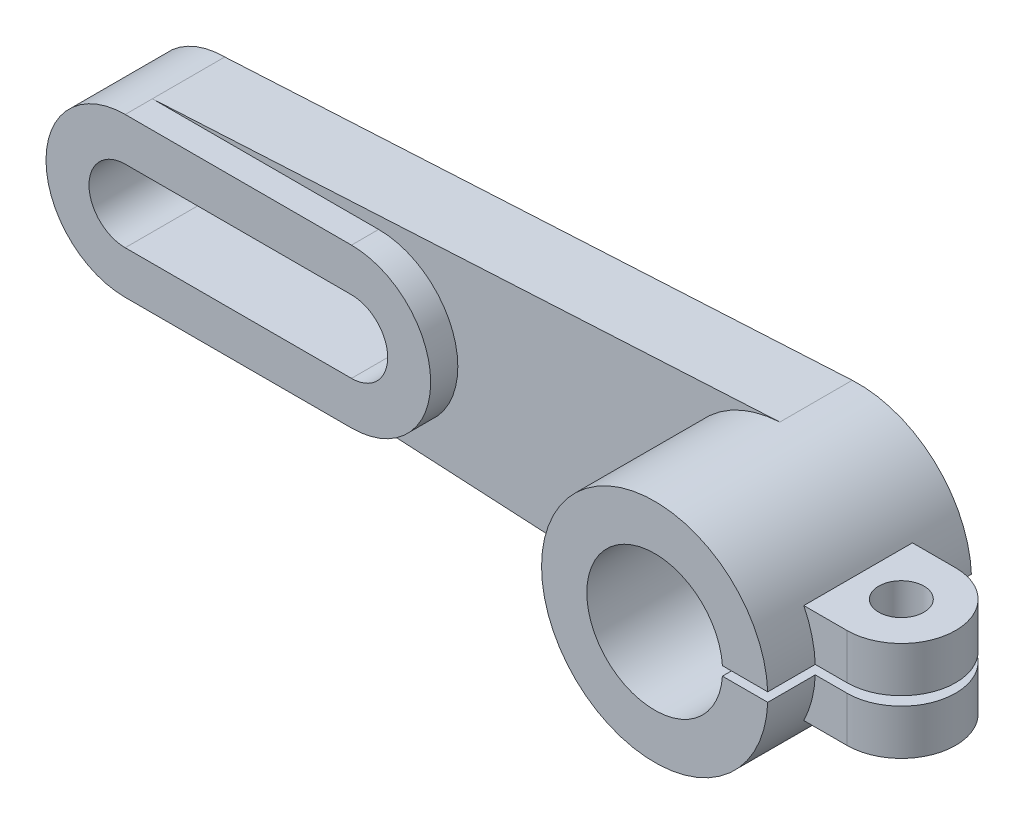
ISO-10303-21;
HEADER;
FILE_DESCRIPTION(('STEP AP214'),'2;1');
FILE_NAME('part.step','',(''),(''),'','','');
FILE_SCHEMA(('AUTOMOTIVE_DESIGN { 1 0 10303 214 1 1 1 1 }'));
ENDSEC;
DATA;
#1=APPLICATION_CONTEXT('core data for automotive mechanical design processes');
#2=APPLICATION_PROTOCOL_DEFINITION('international standard','automotive_design',2000,#1);
#3=PRODUCT_CONTEXT('',#1,'mechanical');
#4=PRODUCT('Part','Part','',(#3));
#5=PRODUCT_RELATED_PRODUCT_CATEGORY('part','',(#4));
#6=PRODUCT_DEFINITION_FORMATION('','',#4);
#7=PRODUCT_DEFINITION_CONTEXT('part definition',#1,'design');
#8=PRODUCT_DEFINITION('design','',#6,#7);
#9=PRODUCT_DEFINITION_SHAPE('','',#8);
#10=(LENGTH_UNIT() NAMED_UNIT(*) SI_UNIT(.MILLI.,.METRE.));
#11=(NAMED_UNIT(*) PLANE_ANGLE_UNIT() SI_UNIT($,.RADIAN.));
#12=(NAMED_UNIT(*) SI_UNIT($,.STERADIAN.) SOLID_ANGLE_UNIT());
#13=UNCERTAINTY_MEASURE_WITH_UNIT(LENGTH_MEASURE(1.E-05),#10,'distance_accuracy_value','');
#14=(GEOMETRIC_REPRESENTATION_CONTEXT(3) GLOBAL_UNCERTAINTY_ASSIGNED_CONTEXT((#13)) GLOBAL_UNIT_ASSIGNED_CONTEXT((#10,
#11,#12)) REPRESENTATION_CONTEXT('',''));
#15=CARTESIAN_POINT('',(0.,0.,0.));
#16=DIRECTION('',(0.,0.,1.));
#17=DIRECTION('',(1.,0.,0.));
#18=AXIS2_PLACEMENT_3D('',#15,#16,#17);
#19=CARTESIAN_POINT('',(32.,11.,22.5));
#20=DIRECTION('',(0.,-1.,0.));
#21=DIRECTION('',(0.,0.,-1.));
#22=AXIS2_PLACEMENT_3D('',#19,#20,#21);
#23=CYLINDRICAL_SURFACE('',#22,12.);
#24=DIRECTION('',(0.,-1.,0.));
#25=VECTOR('',#24,1.);
#26=CARTESIAN_POINT('',(32.,11.,10.5));
#27=LINE('',#26,#25);
#28=CARTESIAN_POINT('',(32.,-1.,10.5));
#29=VERTEX_POINT('',#28);
#30=CARTESIAN_POINT('',(32.,-11.,10.5));
#31=VERTEX_POINT('',#30);
#32=EDGE_CURVE('E301',#29,#31,#27,.T.);
#33=ORIENTED_EDGE('',*,*,#32,.F.);
#34=CARTESIAN_POINT('',(32.,-1.,22.5));
#35=DIRECTION('',(0.,-1.,0.));
#36=DIRECTION('',(0.,0.,-1.));
#37=AXIS2_PLACEMENT_3D('',#34,#35,#36);
#38=CIRCLE('',#37,12.);
#39=CARTESIAN_POINT('',(32.,-1.,34.5));
#40=VERTEX_POINT('',#39);
#41=EDGE_CURVE('E267',#29,#40,#38,.T.);
#42=ORIENTED_EDGE('',*,*,#41,.T.);
#43=DIRECTION('',(0.,-1.,0.));
#44=VECTOR('',#43,1.);
#45=CARTESIAN_POINT('',(32.,11.,34.5));
#46=LINE('',#45,#44);
#47=CARTESIAN_POINT('',(32.,-11.,34.5));
#48=VERTEX_POINT('',#47);
#49=EDGE_CURVE('E291',#40,#48,#46,.T.);
#50=ORIENTED_EDGE('',*,*,#49,.T.);
#51=CARTESIAN_POINT('',(32.,-11.,22.5));
#52=DIRECTION('',(0.,1.,0.));
#53=DIRECTION('',(0.,0.,1.));
#54=AXIS2_PLACEMENT_3D('',#51,#52,#53);
#55=CIRCLE('',#54,12.);
#56=EDGE_CURVE('E278',#48,#31,#55,.T.);
#57=ORIENTED_EDGE('',*,*,#56,.T.);
#58=EDGE_LOOP('',(#33,#42,#50,#57));
#59=FACE_BOUND('',#58,.T.);
#60=ADVANCED_FACE('F43',(#59),#23,.T.);
#61=CARTESIAN_POINT('',(16.6767998289148,11.,10.5));
#62=DIRECTION('',(0.,0.,1.));
#63=DIRECTION('',(1.,0.,0.));
#64=AXIS2_PLACEMENT_3D('',#61,#62,#63);
#65=PLANE('',#64);
#66=CARTESIAN_POINT('',(0.,0.,10.5));
#67=DIRECTION('',(0.,0.,1.));
#68=DIRECTION('',(1.,0.,0.));
#69=AXIS2_PLACEMENT_3D('',#66,#67,#68);
#70=CIRCLE('',#69,25.);
#71=CARTESIAN_POINT('',(22.4499443206436,-11.,10.5));
#72=VERTEX_POINT('',#71);
#73=CARTESIAN_POINT('',(24.9799919935936,-1.,10.5));
#74=VERTEX_POINT('',#73);
#75=EDGE_CURVE('E11',#72,#74,#70,.T.);
#76=ORIENTED_EDGE('',*,*,#75,.T.);
#77=DIRECTION('',(1.,0.,0.));
#78=VECTOR('',#77,1.);
#79=CARTESIAN_POINT('',(16.6767998289148,-1.,10.5));
#80=LINE('',#79,#78);
#81=EDGE_CURVE('E272',#74,#29,#80,.T.);
#82=ORIENTED_EDGE('',*,*,#81,.T.);
#83=ORIENTED_EDGE('',*,*,#32,.T.);
#84=DIRECTION('',(-1.,0.,0.));
#85=VECTOR('',#84,1.);
#86=CARTESIAN_POINT('',(16.6767998289148,-11.,10.5));
#87=LINE('',#86,#85);
#88=EDGE_CURVE('E298',#31,#72,#87,.T.);
#89=ORIENTED_EDGE('',*,*,#88,.T.);
#90=EDGE_LOOP('',(#76,#82,#83,#89));
#91=FACE_BOUND('',#90,.T.);
#92=ADVANCED_FACE('F411',(#91),#65,.F.);
#93=CARTESIAN_POINT('',(32.,11.,34.5));
#94=DIRECTION('',(0.,0.,-1.));
#95=DIRECTION('',(-1.,0.,0.));
#96=AXIS2_PLACEMENT_3D('',#93,#94,#95);
#97=PLANE('',#96);
#98=ORIENTED_EDGE('',*,*,#49,.F.);
#99=DIRECTION('',(-1.,0.,0.));
#100=VECTOR('',#99,1.);
#101=CARTESIAN_POINT('',(32.,-1.,34.5));
#102=LINE('',#101,#100);
#103=CARTESIAN_POINT('',(24.9799919935936,-1.,34.5));
#104=VERTEX_POINT('',#103);
#105=EDGE_CURVE('E270',#40,#104,#102,.T.);
#106=ORIENTED_EDGE('',*,*,#105,.T.);
#107=CARTESIAN_POINT('',(0.,0.,34.5));
#108=DIRECTION('',(0.,0.,-1.));
#109=DIRECTION('',(-1.,0.,0.));
#110=AXIS2_PLACEMENT_3D('',#107,#108,#109);
#111=CIRCLE('',#110,25.);
#112=CARTESIAN_POINT('',(22.4499443206436,-11.,34.5));
#113=VERTEX_POINT('',#112);
#114=EDGE_CURVE('E237',#104,#113,#111,.T.);
#115=ORIENTED_EDGE('',*,*,#114,.T.);
#116=DIRECTION('',(1.,0.,0.));
#117=VECTOR('',#116,1.);
#118=CARTESIAN_POINT('',(32.,-11.,34.5));
#119=LINE('',#118,#117);
#120=EDGE_CURVE('E289',#113,#48,#119,.T.);
#121=ORIENTED_EDGE('',*,*,#120,.T.);
#122=EDGE_LOOP('',(#98,#106,#115,#121));
#123=FACE_BOUND('',#122,.T.);
#124=ADVANCED_FACE('F425',(#123),#97,.F.);
#125=CARTESIAN_POINT('',(32.,11.,22.5));
#126=DIRECTION('',(0.,-1.,0.));
#127=DIRECTION('',(0.,0.,-1.));
#128=AXIS2_PLACEMENT_3D('',#125,#126,#127);
#129=CYLINDRICAL_SURFACE('',#128,5.);
#130=CARTESIAN_POINT('',(32.,-1.,22.5));
#131=DIRECTION('',(0.,-1.,0.));
#132=DIRECTION('',(0.,0.,-1.));
#133=AXIS2_PLACEMENT_3D('',#130,#131,#132);
#134=CIRCLE('',#133,5.);
#135=CARTESIAN_POINT('',(32.,-1.,17.5));
#136=VERTEX_POINT('',#135);
#137=EDGE_CURVE('E50',#136,#136,#134,.T.);
#138=ORIENTED_EDGE('',*,*,#137,.F.);
#139=EDGE_LOOP('',(#138));
#140=FACE_BOUND('',#139,.T.);
#141=CARTESIAN_POINT('',(32.,-11.,22.5));
#142=DIRECTION('',(0.,1.,0.));
#143=DIRECTION('',(0.,0.,1.));
#144=AXIS2_PLACEMENT_3D('',#141,#142,#143);
#145=CIRCLE('',#144,5.);
#146=CARTESIAN_POINT('',(32.,-11.,27.5));
#147=VERTEX_POINT('',#146);
#148=EDGE_CURVE('E283',#147,#147,#145,.T.);
#149=ORIENTED_EDGE('',*,*,#148,.F.);
#150=EDGE_LOOP('',(#149));
#151=FACE_BOUND('',#150,.T.);
#152=ADVANCED_FACE('F412',(#140,#151),#129,.F.);
#153=CARTESIAN_POINT('',(0.,0.,45.));
#154=DIRECTION('',(0.,0.,-1.));
#155=DIRECTION('',(-1.,0.,0.));
#156=AXIS2_PLACEMENT_3D('',#153,#154,#155);
#157=CYLINDRICAL_SURFACE('',#156,25.);
#158=CARTESIAN_POINT('',(0.,0.,0.));
#159=DIRECTION('',(0.,0.,1.));
#160=DIRECTION('',(1.,0.,0.));
#161=AXIS2_PLACEMENT_3D('',#158,#159,#160);
#162=CIRCLE('',#161,25.);
#163=CARTESIAN_POINT('',(-2.67090620031804,-24.8569157392687,0.));
#164=VERTEX_POINT('',#163);
#165=CARTESIAN_POINT('',(24.9799919935936,-1.,0.));
#166=VERTEX_POINT('',#165);
#167=EDGE_CURVE('E240',#164,#166,#162,.T.);
#168=ORIENTED_EDGE('',*,*,#167,.T.);
#169=DIRECTION('',(0.,0.,-1.));
#170=VECTOR('',#169,1.);
#171=CARTESIAN_POINT('',(24.9799919935936,-1.,45.));
#172=LINE('',#171,#170);
#173=EDGE_CURVE('E273',#166,#74,#172,.F.);
#174=ORIENTED_EDGE('',*,*,#173,.T.);
#175=ORIENTED_EDGE('',*,*,#75,.F.);
#176=DIRECTION('',(0.,0.,-1.));
#177=VECTOR('',#176,1.);
#178=CARTESIAN_POINT('',(22.4499443206436,-11.,45.));
#179=LINE('',#178,#177);
#180=EDGE_CURVE('E241',#113,#72,#179,.T.);
#181=ORIENTED_EDGE('',*,*,#180,.F.);
#182=ORIENTED_EDGE('',*,*,#114,.F.);
#183=CARTESIAN_POINT('',(24.9799919935936,-1.,45.));
#184=VERTEX_POINT('',#183);
#185=EDGE_CURVE('E69',#104,#184,#172,.F.);
#186=ORIENTED_EDGE('',*,*,#185,.T.);
#187=CARTESIAN_POINT('',(0.,0.,45.));
#188=DIRECTION('',(0.,0.,1.));
#189=DIRECTION('',(1.,0.,0.));
#190=AXIS2_PLACEMENT_3D('',#187,#188,#189);
#191=CIRCLE('',#190,25.);
#192=CARTESIAN_POINT('',(24.9799919935936,1.,45.));
#193=VERTEX_POINT('',#192);
#194=EDGE_CURVE('E234',#193,#184,#191,.T.);
#195=ORIENTED_EDGE('',*,*,#194,.F.);
#196=DIRECTION('',(0.,0.,-1.));
#197=VECTOR('',#196,1.);
#198=CARTESIAN_POINT('',(24.9799919935936,1.,45.));
#199=LINE('',#198,#197);
#200=CARTESIAN_POINT('',(24.9799919935936,1.,34.5));
#201=VERTEX_POINT('',#200);
#202=EDGE_CURVE('E257',#193,#201,#199,.T.);
#203=ORIENTED_EDGE('',*,*,#202,.T.);
#204=CARTESIAN_POINT('',(22.4499443206436,11.,34.5));
#205=VERTEX_POINT('',#204);
#206=EDGE_CURVE('E238',#205,#201,#111,.T.);
#207=ORIENTED_EDGE('',*,*,#206,.F.);
#208=DIRECTION('',(0.,0.,-1.));
#209=VECTOR('',#208,1.);
#210=CARTESIAN_POINT('',(22.4499443206436,11.,45.));
#211=LINE('',#210,#209);
#212=CARTESIAN_POINT('',(22.4499443206436,11.,10.5));
#213=VERTEX_POINT('',#212);
#214=EDGE_CURVE('E247',#205,#213,#211,.T.);
#215=ORIENTED_EDGE('',*,*,#214,.T.);
#216=CARTESIAN_POINT('',(24.9799919935936,1.,10.5));
#217=VERTEX_POINT('',#216);
#218=EDGE_CURVE('E55',#217,#213,#70,.T.);
#219=ORIENTED_EDGE('',*,*,#218,.F.);
#220=CARTESIAN_POINT('',(24.9799919935936,1.,0.));
#221=VERTEX_POINT('',#220);
#222=EDGE_CURVE('E262',#217,#221,#199,.T.);
#223=ORIENTED_EDGE('',*,*,#222,.T.);
#224=CARTESIAN_POINT('',(-1.3438034995607,24.9638577178001,0.));
#225=VERTEX_POINT('',#224);
#226=EDGE_CURVE('E219',#221,#225,#162,.T.);
#227=ORIENTED_EDGE('',*,*,#226,.T.);
#228=DIRECTION('',(0.,0.,-1.));
#229=VECTOR('',#228,1.);
#230=CARTESIAN_POINT('',(-1.3438034995607,24.9638577178001,16.));
#231=LINE('',#230,#229);
#232=CARTESIAN_POINT('',(-1.3438034995607,24.9638577178001,16.));
#233=VERTEX_POINT('',#232);
#234=EDGE_CURVE('E383',#233,#225,#231,.T.);
#235=ORIENTED_EDGE('',*,*,#234,.F.);
#236=CARTESIAN_POINT('',(0.,0.,16.));
#237=DIRECTION('',(0.,0.,1.));
#238=DIRECTION('',(1.,0.,0.));
#239=AXIS2_PLACEMENT_3D('',#236,#237,#238);
#240=CIRCLE('',#239,25.);
#241=CARTESIAN_POINT('',(-2.67090620031804,-24.8569157392687,16.));
#242=VERTEX_POINT('',#241);
#243=EDGE_CURVE('E372',#233,#242,#240,.T.);
#244=ORIENTED_EDGE('',*,*,#243,.T.);
#245=DIRECTION('',(0.,0.,-1.));
#246=VECTOR('',#245,1.);
#247=CARTESIAN_POINT('',(-2.67090620031804,-24.8569157392687,16.));
#248=LINE('',#247,#246);
#249=EDGE_CURVE('E229',#242,#164,#248,.T.);
#250=ORIENTED_EDGE('',*,*,#249,.T.);
#251=EDGE_LOOP('',(#168,#174,#175,#181,#182,#186,#195,#203,#207,#215,#219,#223,#227,#235,#244,#250));
#252=FACE_BOUND('',#251,.T.);
#253=ADVANCED_FACE('F44',(#252),#157,.T.);
#254=CARTESIAN_POINT('',(0.,0.,45.));
#255=DIRECTION('',(0.,0.,1.));
#256=DIRECTION('',(1.,0.,0.));
#257=AXIS2_PLACEMENT_3D('',#254,#255,#256);
#258=PLANE('',#257);
#259=DIRECTION('',(1.,0.,0.));
#260=VECTOR('',#259,1.);
#261=CARTESIAN_POINT('',(47.1313441008684,-1.,45.));
#262=LINE('',#261,#260);
#263=CARTESIAN_POINT('',(14.9666295470958,-1.,45.));
#264=VERTEX_POINT('',#263);
#265=EDGE_CURVE('E222',#264,#184,#262,.T.);
#266=ORIENTED_EDGE('',*,*,#265,.F.);
#267=CARTESIAN_POINT('',(0.,0.,45.));
#268=DIRECTION('',(0.,0.,1.));
#269=DIRECTION('',(1.,0.,0.));
#270=AXIS2_PLACEMENT_3D('',#267,#268,#269);
#271=CIRCLE('',#270,15.);
#272=CARTESIAN_POINT('',(14.9666295470958,1.,45.));
#273=VERTEX_POINT('',#272);
#274=EDGE_CURVE('E223',#273,#264,#271,.T.);
#275=ORIENTED_EDGE('',*,*,#274,.F.);
#276=DIRECTION('',(-1.,0.,0.));
#277=VECTOR('',#276,1.);
#278=CARTESIAN_POINT('',(14.9666295470958,1.,45.));
#279=LINE('',#278,#277);
#280=EDGE_CURVE('E204',#193,#273,#279,.T.);
#281=ORIENTED_EDGE('',*,*,#280,.F.);
#282=ORIENTED_EDGE('',*,*,#194,.T.);
#283=EDGE_LOOP('',(#266,#275,#281,#282));
#284=FACE_BOUND('',#283,.T.);
#285=ADVANCED_FACE('F404',(#284),#258,.T.);
#286=CARTESIAN_POINT('',(0.,0.,0.));
#287=DIRECTION('',(0.,0.,1.));
#288=DIRECTION('',(1.,0.,0.));
#289=AXIS2_PLACEMENT_3D('',#286,#287,#288);
#290=PLANE('',#289);
#291=CARTESIAN_POINT('',(0.,0.,0.));
#292=DIRECTION('',(0.,0.,1.));
#293=DIRECTION('',(1.,0.,0.));
#294=AXIS2_PLACEMENT_3D('',#291,#292,#293);
#295=CIRCLE('',#294,15.);
#296=CARTESIAN_POINT('',(14.9666295470958,1.,0.));
#297=VERTEX_POINT('',#296);
#298=CARTESIAN_POINT('',(14.9666295470958,-1.,0.));
#299=VERTEX_POINT('',#298);
#300=EDGE_CURVE('E217',#297,#299,#295,.T.);
#301=ORIENTED_EDGE('',*,*,#300,.T.);
#302=DIRECTION('',(1.,0.,0.));
#303=VECTOR('',#302,1.);
#304=CARTESIAN_POINT('',(14.9666295470958,-1.,0.));
#305=LINE('',#304,#303);
#306=EDGE_CURVE('E209',#299,#166,#305,.T.);
#307=ORIENTED_EDGE('',*,*,#306,.T.);
#308=ORIENTED_EDGE('',*,*,#167,.F.);
#309=DIRECTION('',(0.998568132270089,-0.0534947213716118,0.));
#310=VECTOR('',#309,1.);
#311=CARTESIAN_POINT('',(-1.33545310015898,-24.9284578696343,0.));
#312=LINE('',#311,#310);
#313=CARTESIAN_POINT('',(-140.,-17.5,0.));
#314=VERTEX_POINT('',#313);
#315=EDGE_CURVE('E363',#314,#164,#312,.T.);
#316=ORIENTED_EDGE('',*,*,#315,.F.);
#317=CARTESIAN_POINT('',(-140.,0.,0.));
#318=DIRECTION('',(0.,0.,1.));
#319=DIRECTION('',(1.,0.,0.));
#320=AXIS2_PLACEMENT_3D('',#317,#318,#319);
#321=CIRCLE('',#320,17.5);
#322=CARTESIAN_POINT('',(-140.,17.5,0.));
#323=VERTEX_POINT('',#322);
#324=EDGE_CURVE('E337',#323,#314,#321,.T.);
#325=ORIENTED_EDGE('',*,*,#324,.F.);
#326=DIRECTION('',(0.998554308712005,0.0537521399824281,0.));
#327=VECTOR('',#326,1.);
#328=CARTESIAN_POINT('',(-1.3438034995607,24.9638577178001,0.));
#329=LINE('',#328,#327);
#330=EDGE_CURVE('E368',#323,#225,#329,.T.);
#331=ORIENTED_EDGE('',*,*,#330,.T.);
#332=ORIENTED_EDGE('',*,*,#226,.F.);
#333=DIRECTION('',(-1.,0.,0.));
#334=VECTOR('',#333,1.);
#335=CARTESIAN_POINT('',(43.9273116343927,1.,0.));
#336=LINE('',#335,#334);
#337=EDGE_CURVE('E203',#221,#297,#336,.T.);
#338=ORIENTED_EDGE('',*,*,#337,.T.);
#339=EDGE_LOOP('',(#301,#307,#308,#316,#325,#331,#332,#338));
#340=FACE_BOUND('',#339,.T.);
#341=CARTESIAN_POINT('',(-140.,0.,0.));
#342=DIRECTION('',(0.,0.,1.));
#343=DIRECTION('',(1.,0.,0.));
#344=AXIS2_PLACEMENT_3D('',#341,#342,#343);
#345=CIRCLE('',#344,8.);
#346=CARTESIAN_POINT('',(-140.,7.99999999999998,0.));
#347=VERTEX_POINT('',#346);
#348=CARTESIAN_POINT('',(-140.,-8.00000000000002,0.));
#349=VERTEX_POINT('',#348);
#350=EDGE_CURVE('E306',#347,#349,#345,.T.);
#351=ORIENTED_EDGE('',*,*,#350,.T.);
#352=DIRECTION('',(1.,0.,0.));
#353=VECTOR('',#352,1.);
#354=CARTESIAN_POINT('',(-140.,-8.00000000000002,0.));
#355=LINE('',#354,#353);
#356=CARTESIAN_POINT('',(-90.,-8.,0.));
#357=VERTEX_POINT('',#356);
#358=EDGE_CURVE('E325',#349,#357,#355,.T.);
#359=ORIENTED_EDGE('',*,*,#358,.T.);
#360=CARTESIAN_POINT('',(-90.,0.,0.));
#361=DIRECTION('',(0.,0.,1.));
#362=DIRECTION('',(1.,0.,0.));
#363=AXIS2_PLACEMENT_3D('',#360,#361,#362);
#364=CIRCLE('',#363,8.);
#365=CARTESIAN_POINT('',(-90.,7.99999999999998,0.));
#366=VERTEX_POINT('',#365);
#367=EDGE_CURVE('E324',#357,#366,#364,.T.);
#368=ORIENTED_EDGE('',*,*,#367,.T.);
#369=DIRECTION('',(-1.,0.,0.));
#370=VECTOR('',#369,1.);
#371=CARTESIAN_POINT('',(-140.,7.99999999999998,0.));
#372=LINE('',#371,#370);
#373=EDGE_CURVE('E315',#366,#347,#372,.T.);
#374=ORIENTED_EDGE('',*,*,#373,.T.);
#375=EDGE_LOOP('',(#351,#359,#368,#374));
#376=FACE_BOUND('',#375,.T.);
#377=ADVANCED_FACE('F214',(#340,#376),#290,.F.);
#378=CARTESIAN_POINT('',(0.,0.,45.));
#379=DIRECTION('',(0.,0.,-1.));
#380=DIRECTION('',(-1.,0.,0.));
#381=AXIS2_PLACEMENT_3D('',#378,#379,#380);
#382=CYLINDRICAL_SURFACE('',#381,15.);
#383=DIRECTION('',(0.,0.,1.));
#384=VECTOR('',#383,1.);
#385=CARTESIAN_POINT('',(14.9666295470958,-1.,0.));
#386=LINE('',#385,#384);
#387=EDGE_CURVE('E207',#299,#264,#386,.T.);
#388=ORIENTED_EDGE('',*,*,#387,.F.);
#389=ORIENTED_EDGE('',*,*,#300,.F.);
#390=DIRECTION('',(0.,0.,1.));
#391=VECTOR('',#390,1.);
#392=CARTESIAN_POINT('',(14.9666295470958,1.,0.));
#393=LINE('',#392,#391);
#394=EDGE_CURVE('E196',#297,#273,#393,.T.);
#395=ORIENTED_EDGE('',*,*,#394,.T.);
#396=ORIENTED_EDGE('',*,*,#274,.T.);
#397=EDGE_LOOP('',(#388,#389,#395,#396));
#398=FACE_BOUND('',#397,.T.);
#399=ADVANCED_FACE('F221',(#398),#382,.F.);
#400=CARTESIAN_POINT('',(-1.33545310015898,-24.9284578696343,16.));
#401=DIRECTION('',(0.0534947213716118,0.998568132270089,0.));
#402=DIRECTION('',(-0.998568132270089,0.0534947213716118,0.));
#403=AXIS2_PLACEMENT_3D('',#400,#401,#402);
#404=PLANE('',#403);
#405=ORIENTED_EDGE('',*,*,#315,.T.);
#406=ORIENTED_EDGE('',*,*,#249,.F.);
#407=DIRECTION('',(0.998568132270089,-0.0534947213716118,0.));
#408=VECTOR('',#407,1.);
#409=CARTESIAN_POINT('',(-1.33545310015898,-24.9284578696343,16.));
#410=LINE('',#409,#408);
#411=CARTESIAN_POINT('',(-140.,-17.5,16.));
#412=VERTEX_POINT('',#411);
#413=EDGE_CURVE('E371',#412,#242,#410,.T.);
#414=ORIENTED_EDGE('',*,*,#413,.F.);
#415=DIRECTION('',(0.,0.,-1.));
#416=VECTOR('',#415,1.);
#417=CARTESIAN_POINT('',(-140.,-17.5,16.));
#418=LINE('',#417,#416);
#419=EDGE_CURVE('E228',#412,#314,#418,.T.);
#420=ORIENTED_EDGE('',*,*,#419,.T.);
#421=EDGE_LOOP('',(#405,#406,#414,#420));
#422=FACE_BOUND('',#421,.T.);
#423=ADVANCED_FACE('F394',(#422),#404,.F.);
#424=CARTESIAN_POINT('',(-1.3438034995607,24.9638577178001,16.));
#425=DIRECTION('',(-0.0537521399824281,0.998554308712005,0.));
#426=DIRECTION('',(-0.998554308712005,-0.0537521399824281,0.));
#427=AXIS2_PLACEMENT_3D('',#424,#425,#426);
#428=PLANE('',#427);
#429=ORIENTED_EDGE('',*,*,#330,.F.);
#430=DIRECTION('',(0.,0.,-1.));
#431=VECTOR('',#430,1.);
#432=CARTESIAN_POINT('',(-140.,17.5,16.));
#433=LINE('',#432,#431);
#434=CARTESIAN_POINT('',(-140.,17.5,16.));
#435=VERTEX_POINT('',#434);
#436=EDGE_CURVE('E377',#435,#323,#433,.T.);
#437=ORIENTED_EDGE('',*,*,#436,.F.);
#438=DIRECTION('',(0.998554308712005,0.0537521399824281,0.));
#439=VECTOR('',#438,1.);
#440=CARTESIAN_POINT('',(-1.3438034995607,24.9638577178001,16.));
#441=LINE('',#440,#439);
#442=EDGE_CURVE('E376',#435,#233,#441,.T.);
#443=ORIENTED_EDGE('',*,*,#442,.T.);
#444=ORIENTED_EDGE('',*,*,#234,.T.);
#445=EDGE_LOOP('',(#429,#437,#443,#444));
#446=FACE_BOUND('',#445,.T.);
#447=ADVANCED_FACE('F528',(#446),#428,.T.);
#448=CARTESIAN_POINT('',(0.,0.,16.));
#449=DIRECTION('',(0.,0.,1.));
#450=DIRECTION('',(1.,0.,0.));
#451=AXIS2_PLACEMENT_3D('',#448,#449,#450);
#452=PLANE('',#451);
#453=DIRECTION('',(1.,0.,0.));
#454=VECTOR('',#453,1.);
#455=CARTESIAN_POINT('',(0.,17.5,16.));
#456=LINE('',#455,#454);
#457=CARTESIAN_POINT('',(-90.,17.5,16.));
#458=VERTEX_POINT('',#457);
#459=EDGE_CURVE('E362',#435,#458,#456,.T.);
#460=ORIENTED_EDGE('',*,*,#459,.T.);
#461=CARTESIAN_POINT('',(-90.,0.,16.));
#462=DIRECTION('',(0.,0.,1.));
#463=DIRECTION('',(1.,0.,0.));
#464=AXIS2_PLACEMENT_3D('',#461,#462,#463);
#465=CIRCLE('',#464,17.5);
#466=CARTESIAN_POINT('',(-90.,-17.5,16.));
#467=VERTEX_POINT('',#466);
#468=EDGE_CURVE('E364',#458,#467,#465,.F.);
#469=ORIENTED_EDGE('',*,*,#468,.T.);
#470=DIRECTION('',(1.,0.,0.));
#471=VECTOR('',#470,1.);
#472=CARTESIAN_POINT('',(0.,-17.5,16.));
#473=LINE('',#472,#471);
#474=EDGE_CURVE('E369',#412,#467,#473,.T.);
#475=ORIENTED_EDGE('',*,*,#474,.F.);
#476=ORIENTED_EDGE('',*,*,#413,.T.);
#477=ORIENTED_EDGE('',*,*,#243,.F.);
#478=ORIENTED_EDGE('',*,*,#442,.F.);
#479=EDGE_LOOP('',(#460,#469,#475,#476,#477,#478));
#480=FACE_BOUND('',#479,.T.);
#481=ADVANCED_FACE('F509',(#480),#452,.T.);
#482=CARTESIAN_POINT('',(-140.,0.,22.));
#483=DIRECTION('',(0.,0.,1.));
#484=DIRECTION('',(1.,0.,0.));
#485=AXIS2_PLACEMENT_3D('',#482,#483,#484);
#486=PLANE('',#485);
#487=CARTESIAN_POINT('',(-140.,0.,22.));
#488=DIRECTION('',(0.,0.,1.));
#489=DIRECTION('',(1.,0.,0.));
#490=AXIS2_PLACEMENT_3D('',#487,#488,#489);
#491=CIRCLE('',#490,17.5);
#492=CARTESIAN_POINT('',(-140.,17.5,22.));
#493=VERTEX_POINT('',#492);
#494=CARTESIAN_POINT('',(-140.,-17.5,22.));
#495=VERTEX_POINT('',#494);
#496=EDGE_CURVE('E339',#493,#495,#491,.T.);
#497=ORIENTED_EDGE('',*,*,#496,.T.);
#498=DIRECTION('',(1.,0.,0.));
#499=VECTOR('',#498,1.);
#500=CARTESIAN_POINT('',(-140.,-17.5,22.));
#501=LINE('',#500,#499);
#502=CARTESIAN_POINT('',(-90.,-17.5,22.));
#503=VERTEX_POINT('',#502);
#504=EDGE_CURVE('E344',#495,#503,#501,.T.);
#505=ORIENTED_EDGE('',*,*,#504,.T.);
#506=CARTESIAN_POINT('',(-90.,0.,22.));
#507=DIRECTION('',(0.,0.,1.));
#508=DIRECTION('',(1.,0.,0.));
#509=AXIS2_PLACEMENT_3D('',#506,#507,#508);
#510=CIRCLE('',#509,17.5);
#511=CARTESIAN_POINT('',(-90.,17.5,22.));
#512=VERTEX_POINT('',#511);
#513=EDGE_CURVE('E343',#503,#512,#510,.T.);
#514=ORIENTED_EDGE('',*,*,#513,.T.);
#515=DIRECTION('',(-1.,0.,0.));
#516=VECTOR('',#515,1.);
#517=CARTESIAN_POINT('',(-140.,17.5,22.));
#518=LINE('',#517,#516);
#519=EDGE_CURVE('E350',#512,#493,#518,.T.);
#520=ORIENTED_EDGE('',*,*,#519,.T.);
#521=EDGE_LOOP('',(#497,#505,#514,#520));
#522=FACE_BOUND('',#521,.T.);
#523=DIRECTION('',(1.,0.,0.));
#524=VECTOR('',#523,1.);
#525=CARTESIAN_POINT('',(-140.,-8.00000000000002,22.));
#526=LINE('',#525,#524);
#527=CARTESIAN_POINT('',(-140.,-8.00000000000002,22.));
#528=VERTEX_POINT('',#527);
#529=CARTESIAN_POINT('',(-90.,-8.,22.));
#530=VERTEX_POINT('',#529);
#531=EDGE_CURVE('E313',#528,#530,#526,.T.);
#532=ORIENTED_EDGE('',*,*,#531,.F.);
#533=CARTESIAN_POINT('',(-140.,0.,22.));
#534=DIRECTION('',(0.,0.,1.));
#535=DIRECTION('',(1.,0.,0.));
#536=AXIS2_PLACEMENT_3D('',#533,#534,#535);
#537=CIRCLE('',#536,8.);
#538=CARTESIAN_POINT('',(-140.,7.99999999999998,22.));
#539=VERTEX_POINT('',#538);
#540=EDGE_CURVE('E310',#539,#528,#537,.T.);
#541=ORIENTED_EDGE('',*,*,#540,.F.);
#542=DIRECTION('',(-1.,0.,0.));
#543=VECTOR('',#542,1.);
#544=CARTESIAN_POINT('',(-140.,7.99999999999998,22.));
#545=LINE('',#544,#543);
#546=CARTESIAN_POINT('',(-90.,7.99999999999998,22.));
#547=VERTEX_POINT('',#546);
#548=EDGE_CURVE('E320',#547,#539,#545,.T.);
#549=ORIENTED_EDGE('',*,*,#548,.F.);
#550=CARTESIAN_POINT('',(-90.,0.,22.));
#551=DIRECTION('',(0.,0.,1.));
#552=DIRECTION('',(1.,0.,0.));
#553=AXIS2_PLACEMENT_3D('',#550,#551,#552);
#554=CIRCLE('',#553,8.);
#555=EDGE_CURVE('E314',#530,#547,#554,.T.);
#556=ORIENTED_EDGE('',*,*,#555,.F.);
#557=EDGE_LOOP('',(#532,#541,#549,#556));
#558=FACE_BOUND('',#557,.T.);
#559=ADVANCED_FACE('F502',(#522,#558),#486,.T.);
#560=CARTESIAN_POINT('',(-140.,0.,22.));
#561=DIRECTION('',(0.,0.,-1.));
#562=DIRECTION('',(-1.,0.,0.));
#563=AXIS2_PLACEMENT_3D('',#560,#561,#562);
#564=CYLINDRICAL_SURFACE('',#563,17.5);
#565=ORIENTED_EDGE('',*,*,#324,.T.);
#566=ORIENTED_EDGE('',*,*,#419,.F.);
#567=DIRECTION('',(0.,0.,-1.));
#568=VECTOR('',#567,1.);
#569=CARTESIAN_POINT('',(-140.,-17.5,22.));
#570=LINE('',#569,#568);
#571=EDGE_CURVE('E359',#495,#412,#570,.T.);
#572=ORIENTED_EDGE('',*,*,#571,.F.);
#573=ORIENTED_EDGE('',*,*,#496,.F.);
#574=DIRECTION('',(0.,0.,-1.));
#575=VECTOR('',#574,1.);
#576=CARTESIAN_POINT('',(-140.,17.5,22.));
#577=LINE('',#576,#575);
#578=EDGE_CURVE('E349',#493,#435,#577,.T.);
#579=ORIENTED_EDGE('',*,*,#578,.T.);
#580=ORIENTED_EDGE('',*,*,#436,.T.);
#581=EDGE_LOOP('',(#565,#566,#572,#573,#579,#580));
#582=FACE_BOUND('',#581,.T.);
#583=ADVANCED_FACE('F510',(#582),#564,.T.);
#584=CARTESIAN_POINT('',(-140.,-17.5,22.));
#585=DIRECTION('',(0.,1.,0.));
#586=DIRECTION('',(-1.,0.,0.));
#587=AXIS2_PLACEMENT_3D('',#584,#585,#586);
#588=PLANE('',#587);
#589=ORIENTED_EDGE('',*,*,#474,.T.);
#590=DIRECTION('',(0.,0.,-1.));
#591=VECTOR('',#590,1.);
#592=CARTESIAN_POINT('',(-90.,-17.5,22.));
#593=LINE('',#592,#591);
#594=EDGE_CURVE('E354',#503,#467,#593,.T.);
#595=ORIENTED_EDGE('',*,*,#594,.F.);
#596=ORIENTED_EDGE('',*,*,#504,.F.);
#597=ORIENTED_EDGE('',*,*,#571,.T.);
#598=EDGE_LOOP('',(#589,#595,#596,#597));
#599=FACE_BOUND('',#598,.T.);
#600=ADVANCED_FACE('F518',(#599),#588,.F.);
#601=CARTESIAN_POINT('',(-90.,0.,22.));
#602=DIRECTION('',(0.,0.,-1.));
#603=DIRECTION('',(-1.,0.,0.));
#604=AXIS2_PLACEMENT_3D('',#601,#602,#603);
#605=CYLINDRICAL_SURFACE('',#604,17.5);
#606=ORIENTED_EDGE('',*,*,#468,.F.);
#607=DIRECTION('',(0.,0.,-1.));
#608=VECTOR('',#607,1.);
#609=CARTESIAN_POINT('',(-90.,17.5,22.));
#610=LINE('',#609,#608);
#611=EDGE_CURVE('E351',#512,#458,#610,.T.);
#612=ORIENTED_EDGE('',*,*,#611,.F.);
#613=ORIENTED_EDGE('',*,*,#513,.F.);
#614=ORIENTED_EDGE('',*,*,#594,.T.);
#615=EDGE_LOOP('',(#606,#612,#613,#614));
#616=FACE_BOUND('',#615,.T.);
#617=ADVANCED_FACE('F515',(#616),#605,.T.);
#618=CARTESIAN_POINT('',(-140.,17.5,22.));
#619=DIRECTION('',(0.,-1.,0.));
#620=DIRECTION('',(1.,0.,0.));
#621=AXIS2_PLACEMENT_3D('',#618,#619,#620);
#622=PLANE('',#621);
#623=ORIENTED_EDGE('',*,*,#459,.F.);
#624=ORIENTED_EDGE('',*,*,#578,.F.);
#625=ORIENTED_EDGE('',*,*,#519,.F.);
#626=ORIENTED_EDGE('',*,*,#611,.T.);
#627=EDGE_LOOP('',(#623,#624,#625,#626));
#628=FACE_BOUND('',#627,.T.);
#629=ADVANCED_FACE('F505',(#628),#622,.F.);
#630=CARTESIAN_POINT('',(-140.,0.,22.));
#631=DIRECTION('',(0.,0.,-1.));
#632=DIRECTION('',(-1.,0.,0.));
#633=AXIS2_PLACEMENT_3D('',#630,#631,#632);
#634=CYLINDRICAL_SURFACE('',#633,8.);
#635=ORIENTED_EDGE('',*,*,#350,.F.);
#636=DIRECTION('',(0.,0.,-1.));
#637=VECTOR('',#636,1.);
#638=CARTESIAN_POINT('',(-140.,7.99999999999998,22.));
#639=LINE('',#638,#637);
#640=EDGE_CURVE('E317',#539,#347,#639,.T.);
#641=ORIENTED_EDGE('',*,*,#640,.F.);
#642=ORIENTED_EDGE('',*,*,#540,.T.);
#643=DIRECTION('',(0.,0.,-1.));
#644=VECTOR('',#643,1.);
#645=CARTESIAN_POINT('',(-140.,-8.00000000000002,22.));
#646=LINE('',#645,#644);
#647=EDGE_CURVE('E338',#528,#349,#646,.T.);
#648=ORIENTED_EDGE('',*,*,#647,.T.);
#649=EDGE_LOOP('',(#635,#641,#642,#648));
#650=FACE_BOUND('',#649,.T.);
#651=ADVANCED_FACE('F499',(#650),#634,.F.);
#652=CARTESIAN_POINT('',(-140.,-8.00000000000002,22.));
#653=DIRECTION('',(0.,1.,0.));
#654=DIRECTION('',(0.,0.,1.));
#655=AXIS2_PLACEMENT_3D('',#652,#653,#654);
#656=PLANE('',#655);
#657=ORIENTED_EDGE('',*,*,#358,.F.);
#658=ORIENTED_EDGE('',*,*,#647,.F.);
#659=ORIENTED_EDGE('',*,*,#531,.T.);
#660=DIRECTION('',(0.,0.,-1.));
#661=VECTOR('',#660,1.);
#662=CARTESIAN_POINT('',(-90.,-8.,22.));
#663=LINE('',#662,#661);
#664=EDGE_CURVE('E331',#530,#357,#663,.T.);
#665=ORIENTED_EDGE('',*,*,#664,.T.);
#666=EDGE_LOOP('',(#657,#658,#659,#665));
#667=FACE_BOUND('',#666,.T.);
#668=ADVANCED_FACE('F491',(#667),#656,.T.);
#669=CARTESIAN_POINT('',(-90.,0.,22.));
#670=DIRECTION('',(0.,0.,-1.));
#671=DIRECTION('',(-1.,0.,0.));
#672=AXIS2_PLACEMENT_3D('',#669,#670,#671);
#673=CYLINDRICAL_SURFACE('',#672,8.);
#674=ORIENTED_EDGE('',*,*,#367,.F.);
#675=ORIENTED_EDGE('',*,*,#664,.F.);
#676=ORIENTED_EDGE('',*,*,#555,.T.);
#677=DIRECTION('',(0.,0.,-1.));
#678=VECTOR('',#677,1.);
#679=CARTESIAN_POINT('',(-90.,7.99999999999998,22.));
#680=LINE('',#679,#678);
#681=EDGE_CURVE('E335',#547,#366,#680,.T.);
#682=ORIENTED_EDGE('',*,*,#681,.T.);
#683=EDGE_LOOP('',(#674,#675,#676,#682));
#684=FACE_BOUND('',#683,.T.);
#685=ADVANCED_FACE('F484',(#684),#673,.F.);
#686=CARTESIAN_POINT('',(-140.,7.99999999999998,22.));
#687=DIRECTION('',(0.,-1.,0.));
#688=DIRECTION('',(0.,0.,-1.));
#689=AXIS2_PLACEMENT_3D('',#686,#687,#688);
#690=PLANE('',#689);
#691=ORIENTED_EDGE('',*,*,#373,.F.);
#692=ORIENTED_EDGE('',*,*,#681,.F.);
#693=ORIENTED_EDGE('',*,*,#548,.T.);
#694=ORIENTED_EDGE('',*,*,#640,.T.);
#695=EDGE_LOOP('',(#691,#692,#693,#694));
#696=FACE_BOUND('',#695,.T.);
#697=ADVANCED_FACE('F477',(#696),#690,.T.);
#698=CARTESIAN_POINT('',(32.,11.,22.5));
#699=DIRECTION('',(0.,1.,0.));
#700=DIRECTION('',(0.,0.,1.));
#701=AXIS2_PLACEMENT_3D('',#698,#699,#700);
#702=PLANE('',#701);
#703=CARTESIAN_POINT('',(32.,11.,22.5));
#704=DIRECTION('',(0.,1.,0.));
#705=DIRECTION('',(0.,0.,1.));
#706=AXIS2_PLACEMENT_3D('',#703,#704,#705);
#707=CIRCLE('',#706,5.);
#708=CARTESIAN_POINT('',(32.,11.,27.5));
#709=VERTEX_POINT('',#708);
#710=EDGE_CURVE('E280',#709,#709,#707,.T.);
#711=ORIENTED_EDGE('',*,*,#710,.F.);
#712=EDGE_LOOP('',(#711));
#713=FACE_BOUND('',#712,.T.);
#714=ORIENTED_EDGE('',*,*,#214,.F.);
#715=DIRECTION('',(1.,0.,0.));
#716=VECTOR('',#715,1.);
#717=CARTESIAN_POINT('',(25.,11.,34.5));
#718=LINE('',#717,#716);
#719=CARTESIAN_POINT('',(32.,11.,34.5));
#720=VERTEX_POINT('',#719);
#721=EDGE_CURVE('E292',#205,#720,#718,.T.);
#722=ORIENTED_EDGE('',*,*,#721,.T.);
#723=CARTESIAN_POINT('',(32.,11.,22.5));
#724=DIRECTION('',(0.,1.,0.));
#725=DIRECTION('',(0.,0.,1.));
#726=AXIS2_PLACEMENT_3D('',#723,#724,#725);
#727=CIRCLE('',#726,12.);
#728=CARTESIAN_POINT('',(32.,11.,10.5));
#729=VERTEX_POINT('',#728);
#730=EDGE_CURVE('E282',#720,#729,#727,.T.);
#731=ORIENTED_EDGE('',*,*,#730,.T.);
#732=DIRECTION('',(-1.,0.,0.));
#733=VECTOR('',#732,1.);
#734=CARTESIAN_POINT('',(25.,11.,10.5));
#735=LINE('',#734,#733);
#736=EDGE_CURVE('E290',#729,#213,#735,.T.);
#737=ORIENTED_EDGE('',*,*,#736,.T.);
#738=EDGE_LOOP('',(#714,#722,#731,#737));
#739=FACE_BOUND('',#738,.T.);
#740=ADVANCED_FACE('F440',(#713,#739),#702,.T.);
#741=CARTESIAN_POINT('',(32.,-11.,22.5));
#742=DIRECTION('',(0.,1.,0.));
#743=DIRECTION('',(0.,0.,1.));
#744=AXIS2_PLACEMENT_3D('',#741,#742,#743);
#745=PLANE('',#744);
#746=ORIENTED_EDGE('',*,*,#148,.T.);
#747=EDGE_LOOP('',(#746));
#748=FACE_BOUND('',#747,.T.);
#749=ORIENTED_EDGE('',*,*,#120,.F.);
#750=ORIENTED_EDGE('',*,*,#180,.T.);
#751=ORIENTED_EDGE('',*,*,#88,.F.);
#752=ORIENTED_EDGE('',*,*,#56,.F.);
#753=EDGE_LOOP('',(#749,#750,#751,#752));
#754=FACE_BOUND('',#753,.T.);
#755=ADVANCED_FACE('F427',(#748,#754),#745,.F.);
#756=CARTESIAN_POINT('',(32.,1.,34.5));
#757=VERTEX_POINT('',#756);
#758=EDGE_CURVE('E302',#720,#757,#46,.T.);
#759=ORIENTED_EDGE('',*,*,#758,.T.);
#760=CARTESIAN_POINT('',(32.,1.,22.5));
#761=DIRECTION('',(0.,1.,0.));
#762=DIRECTION('',(0.,0.,1.));
#763=AXIS2_PLACEMENT_3D('',#760,#761,#762);
#764=CIRCLE('',#763,12.);
#765=CARTESIAN_POINT('',(32.,1.,10.5));
#766=VERTEX_POINT('',#765);
#767=EDGE_CURVE('E58',#757,#766,#764,.T.);
#768=ORIENTED_EDGE('',*,*,#767,.T.);
#769=EDGE_CURVE('E303',#729,#766,#27,.T.);
#770=ORIENTED_EDGE('',*,*,#769,.F.);
#771=ORIENTED_EDGE('',*,*,#730,.F.);
#772=EDGE_LOOP('',(#759,#768,#770,#771));
#773=FACE_BOUND('',#772,.T.);
#774=ADVANCED_FACE('F417',(#773),#23,.T.);
#775=ORIENTED_EDGE('',*,*,#769,.T.);
#776=DIRECTION('',(-1.,0.,0.));
#777=VECTOR('',#776,1.);
#778=CARTESIAN_POINT('',(16.6767998289148,1.,10.5));
#779=LINE('',#778,#777);
#780=EDGE_CURVE('E263',#766,#217,#779,.T.);
#781=ORIENTED_EDGE('',*,*,#780,.T.);
#782=ORIENTED_EDGE('',*,*,#218,.T.);
#783=ORIENTED_EDGE('',*,*,#736,.F.);
#784=EDGE_LOOP('',(#775,#781,#782,#783));
#785=FACE_BOUND('',#784,.T.);
#786=ADVANCED_FACE('F422',(#785),#65,.F.);
#787=ORIENTED_EDGE('',*,*,#206,.T.);
#788=DIRECTION('',(1.,0.,0.));
#789=VECTOR('',#788,1.);
#790=CARTESIAN_POINT('',(32.,1.,34.5));
#791=LINE('',#790,#789);
#792=EDGE_CURVE('E248',#201,#757,#791,.T.);
#793=ORIENTED_EDGE('',*,*,#792,.T.);
#794=ORIENTED_EDGE('',*,*,#758,.F.);
#795=ORIENTED_EDGE('',*,*,#721,.F.);
#796=EDGE_LOOP('',(#787,#793,#794,#795));
#797=FACE_BOUND('',#796,.T.);
#798=ADVANCED_FACE('F434',(#797),#97,.F.);
#799=CARTESIAN_POINT('',(32.,1.,22.5));
#800=DIRECTION('',(0.,1.,0.));
#801=DIRECTION('',(0.,0.,1.));
#802=AXIS2_PLACEMENT_3D('',#799,#800,#801);
#803=CIRCLE('',#802,5.);
#804=CARTESIAN_POINT('',(32.,1.,27.5));
#805=VERTEX_POINT('',#804);
#806=EDGE_CURVE('E249',#805,#805,#803,.T.);
#807=ORIENTED_EDGE('',*,*,#806,.F.);
#808=EDGE_LOOP('',(#807));
#809=FACE_BOUND('',#808,.T.);
#810=ORIENTED_EDGE('',*,*,#710,.T.);
#811=EDGE_LOOP('',(#810));
#812=FACE_BOUND('',#811,.T.);
#813=ADVANCED_FACE('F453',(#809,#812),#129,.F.);
#814=CARTESIAN_POINT('',(14.9666295470958,1.,0.));
#815=DIRECTION('',(0.,1.,0.));
#816=DIRECTION('',(0.,0.,1.));
#817=AXIS2_PLACEMENT_3D('',#814,#815,#816);
#818=PLANE('',#817);
#819=ORIENTED_EDGE('',*,*,#806,.T.);
#820=EDGE_LOOP('',(#819));
#821=FACE_BOUND('',#820,.T.);
#822=ORIENTED_EDGE('',*,*,#780,.F.);
#823=ORIENTED_EDGE('',*,*,#767,.F.);
#824=ORIENTED_EDGE('',*,*,#792,.F.);
#825=ORIENTED_EDGE('',*,*,#202,.F.);
#826=ORIENTED_EDGE('',*,*,#280,.T.);
#827=ORIENTED_EDGE('',*,*,#394,.F.);
#828=ORIENTED_EDGE('',*,*,#337,.F.);
#829=ORIENTED_EDGE('',*,*,#222,.F.);
#830=EDGE_LOOP('',(#822,#823,#824,#825,#826,#827,#828,#829));
#831=FACE_BOUND('',#830,.T.);
#832=ADVANCED_FACE('F199',(#821,#831),#818,.F.);
#833=CARTESIAN_POINT('',(47.1313441008684,-1.,0.));
#834=DIRECTION('',(0.,-1.,0.));
#835=DIRECTION('',(0.,0.,-1.));
#836=AXIS2_PLACEMENT_3D('',#833,#834,#835);
#837=PLANE('',#836);
#838=ORIENTED_EDGE('',*,*,#137,.T.);
#839=EDGE_LOOP('',(#838));
#840=FACE_BOUND('',#839,.T.);
#841=ORIENTED_EDGE('',*,*,#306,.F.);
#842=ORIENTED_EDGE('',*,*,#387,.T.);
#843=ORIENTED_EDGE('',*,*,#265,.T.);
#844=ORIENTED_EDGE('',*,*,#185,.F.);
#845=ORIENTED_EDGE('',*,*,#105,.F.);
#846=ORIENTED_EDGE('',*,*,#41,.F.);
#847=ORIENTED_EDGE('',*,*,#81,.F.);
#848=ORIENTED_EDGE('',*,*,#173,.F.);
#849=EDGE_LOOP('',(#841,#842,#843,#844,#845,#846,#847,#848));
#850=FACE_BOUND('',#849,.T.);
#851=ADVANCED_FACE('F396',(#840,#850),#837,.F.);
#852=CLOSED_SHELL('',(#60,#92,#124,#152,#253,#285,#377,#399,#423,#447,#481,#559,#583,#600,#617,
#629,#651,#668,#685,#697,#740,#755,#774,#786,#798,#813,#832,#851));
#853=MANIFOLD_SOLID_BREP('B2',#852);
#854=ADVANCED_BREP_SHAPE_REPRESENTATION('',(#18,#853),#14);
#855=SHAPE_DEFINITION_REPRESENTATION(#9,#854);
ENDSEC;
END-ISO-10303-21;
